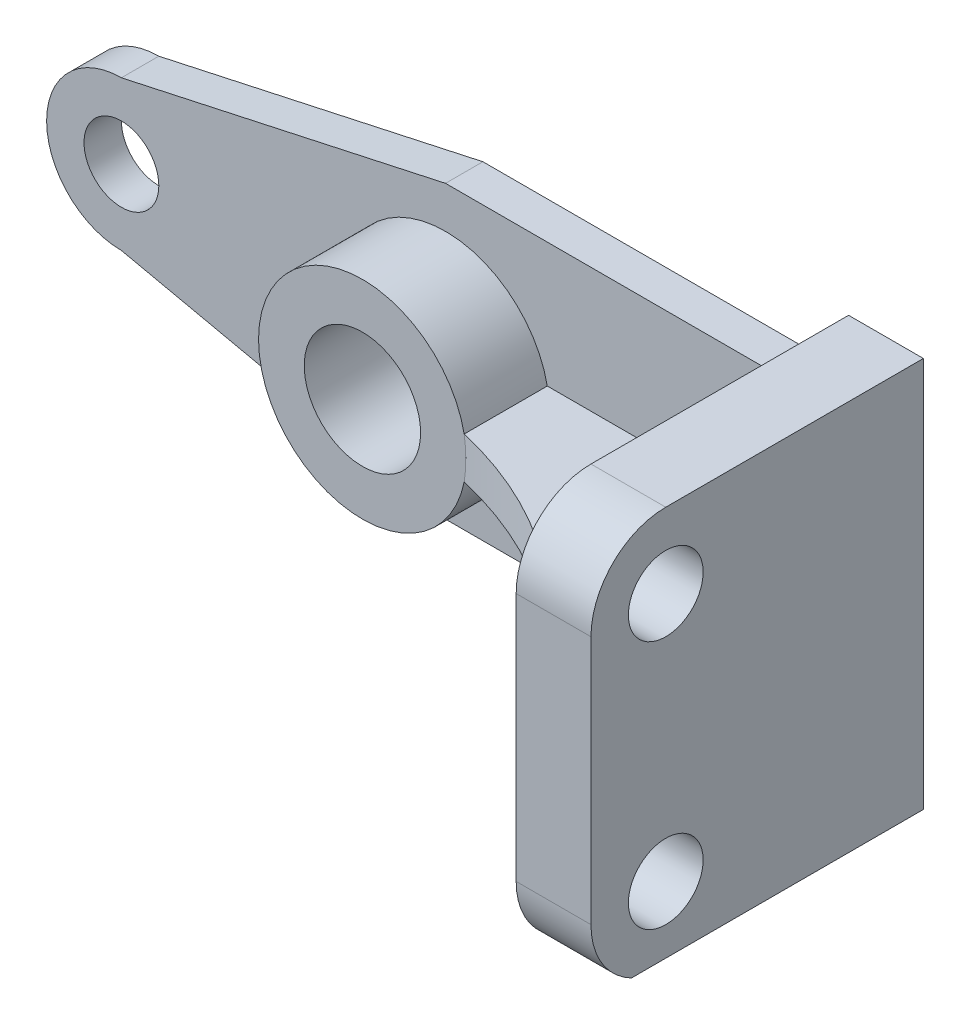
ISO-10303-21;
HEADER;
FILE_DESCRIPTION(('STEP AP214'),'2;1');
FILE_NAME('part.step','',(''),(''),'','','');
FILE_SCHEMA(('AUTOMOTIVE_DESIGN { 1 0 10303 214 1 1 1 1 }'));
ENDSEC;
DATA;
#1=APPLICATION_CONTEXT('core data for automotive mechanical design processes');
#2=APPLICATION_PROTOCOL_DEFINITION('international standard','automotive_design',2000,#1);
#3=PRODUCT_CONTEXT('',#1,'mechanical');
#4=PRODUCT('Part','Part','',(#3));
#5=PRODUCT_RELATED_PRODUCT_CATEGORY('part','',(#4));
#6=PRODUCT_DEFINITION_FORMATION('','',#4);
#7=PRODUCT_DEFINITION_CONTEXT('part definition',#1,'design');
#8=PRODUCT_DEFINITION('design','',#6,#7);
#9=PRODUCT_DEFINITION_SHAPE('','',#8);
#10=(LENGTH_UNIT() NAMED_UNIT(*) SI_UNIT(.MILLI.,.METRE.));
#11=(NAMED_UNIT(*) PLANE_ANGLE_UNIT() SI_UNIT($,.RADIAN.));
#12=(NAMED_UNIT(*) SI_UNIT($,.STERADIAN.) SOLID_ANGLE_UNIT());
#13=UNCERTAINTY_MEASURE_WITH_UNIT(LENGTH_MEASURE(1.E-05),#10,'distance_accuracy_value','');
#14=(GEOMETRIC_REPRESENTATION_CONTEXT(3) GLOBAL_UNCERTAINTY_ASSIGNED_CONTEXT((#13)) GLOBAL_UNIT_ASSIGNED_CONTEXT((#10,
#11,#12)) REPRESENTATION_CONTEXT('',''));
#15=CARTESIAN_POINT('',(0.,0.,0.));
#16=DIRECTION('',(0.,0.,1.));
#17=DIRECTION('',(1.,0.,0.));
#18=AXIS2_PLACEMENT_3D('',#15,#16,#17);
#19=CARTESIAN_POINT('',(88.,-30.9999999999999,62.));
#20=DIRECTION('',(-1.,0.,0.));
#21=DIRECTION('',(0.,0.,1.));
#22=AXIS2_PLACEMENT_3D('',#19,#20,#21);
#23=PLANE('',#22);
#24=CARTESIAN_POINT('',(88.,29.0000000000001,62.));
#25=DIRECTION('',(1.,0.,0.));
#26=DIRECTION('',(0.,0.,-1.));
#27=AXIS2_PLACEMENT_3D('',#24,#25,#26);
#28=CIRCLE('',#27,9.00000000000001);
#29=CARTESIAN_POINT('',(88.,29.0000000000001,53.));
#30=VERTEX_POINT('',#29);
#31=EDGE_CURVE('E407',#30,#30,#28,.T.);
#32=ORIENTED_EDGE('',*,*,#31,.T.);
#33=EDGE_LOOP('',(#32));
#34=FACE_BOUND('',#33,.T.);
#35=DIRECTION('',(0.,1.,0.));
#36=VECTOR('',#35,1.);
#37=CARTESIAN_POINT('',(88.,47.0000000000001,9.));
#38=LINE('',#37,#36);
#39=CARTESIAN_POINT('',(88.,5.,8.99999999999999));
#40=VERTEX_POINT('',#39);
#41=CARTESIAN_POINT('',(88.,47.0000000000001,9.));
#42=VERTEX_POINT('',#41);
#43=EDGE_CURVE('E185',#40,#42,#38,.T.);
#44=ORIENTED_EDGE('',*,*,#43,.F.);
#45=DIRECTION('',(0.,0.,-1.));
#46=VECTOR('',#45,1.);
#47=CARTESIAN_POINT('',(88.,5.,80.));
#48=LINE('',#47,#46);
#49=CARTESIAN_POINT('',(88.,5.,80.));
#50=VERTEX_POINT('',#49);
#51=EDGE_CURVE('E430',#50,#40,#48,.T.);
#52=ORIENTED_EDGE('',*,*,#51,.F.);
#53=DIRECTION('',(0.,-1.,0.));
#54=VECTOR('',#53,1.);
#55=CARTESIAN_POINT('',(88.,29.,80.));
#56=LINE('',#55,#54);
#57=CARTESIAN_POINT('',(88.,29.,80.));
#58=VERTEX_POINT('',#57);
#59=EDGE_CURVE('E392',#58,#50,#56,.T.);
#60=ORIENTED_EDGE('',*,*,#59,.F.);
#61=CARTESIAN_POINT('',(88.,29.0000000000001,62.));
#62=DIRECTION('',(1.,0.,0.));
#63=DIRECTION('',(0.,0.,-1.));
#64=AXIS2_PLACEMENT_3D('',#61,#62,#63);
#65=CIRCLE('',#64,18.);
#66=CARTESIAN_POINT('',(88.,47.0000000000001,61.9999999999999));
#67=VERTEX_POINT('',#66);
#68=EDGE_CURVE('E400',#67,#58,#65,.T.);
#69=ORIENTED_EDGE('',*,*,#68,.F.);
#70=DIRECTION('',(0.,0.,1.));
#71=VECTOR('',#70,1.);
#72=CARTESIAN_POINT('',(88.,47.0000000000001,9.));
#73=LINE('',#72,#71);
#74=EDGE_CURVE('E397',#42,#67,#73,.T.);
#75=ORIENTED_EDGE('',*,*,#74,.F.);
#76=EDGE_LOOP('',(#44,#52,#60,#69,#75));
#77=FACE_BOUND('',#76,.T.);
#78=ADVANCED_FACE('F43',(#34,#77),#23,.T.);
#79=CARTESIAN_POINT('',(0.,0.,9.));
#80=DIRECTION('',(0.,0.,1.));
#81=DIRECTION('',(1.,0.,0.));
#82=AXIS2_PLACEMENT_3D('',#79,#80,#81);
#83=PLANE('',#82);
#84=DIRECTION('',(-1.,0.,0.));
#85=VECTOR('',#84,1.);
#86=CARTESIAN_POINT('',(0.,-5.,9.));
#87=LINE('',#86,#85);
#88=CARTESIAN_POINT('',(88.,-5.,8.99999999999999));
#89=VERTEX_POINT('',#88);
#90=CARTESIAN_POINT('',(24.4948974278318,-5.,9.));
#91=VERTEX_POINT('',#90);
#92=EDGE_CURVE('E431',#89,#91,#87,.T.);
#93=ORIENTED_EDGE('',*,*,#92,.T.);
#94=CARTESIAN_POINT('',(0.,0.,9.));
#95=DIRECTION('',(0.,0.,1.));
#96=DIRECTION('',(1.,0.,0.));
#97=AXIS2_PLACEMENT_3D('',#94,#95,#96);
#98=CIRCLE('',#97,25.);
#99=CARTESIAN_POINT('',(24.4948974278318,5.,9.));
#100=VERTEX_POINT('',#99);
#101=EDGE_CURVE('E420',#100,#91,#98,.T.);
#102=ORIENTED_EDGE('',*,*,#101,.F.);
#103=DIRECTION('',(-1.,0.,0.));
#104=VECTOR('',#103,1.);
#105=CARTESIAN_POINT('',(0.,5.,9.));
#106=LINE('',#105,#104);
#107=EDGE_CURVE('E63',#40,#100,#106,.T.);
#108=ORIENTED_EDGE('',*,*,#107,.F.);
#109=ORIENTED_EDGE('',*,*,#43,.T.);
#110=CARTESIAN_POINT('',(76.,47.,9.));
#111=DIRECTION('',(0.,0.,1.));
#112=DIRECTION('',(1.,0.,0.));
#113=AXIS2_PLACEMENT_3D('',#110,#111,#112);
#114=CIRCLE('',#113,12.);
#115=CARTESIAN_POINT('',(75.9999999999999,35.,9.));
#116=VERTEX_POINT('',#115);
#117=EDGE_CURVE('E345',#116,#42,#114,.T.);
#118=ORIENTED_EDGE('',*,*,#117,.F.);
#119=DIRECTION('',(1.,0.,0.));
#120=VECTOR('',#119,1.);
#121=CARTESIAN_POINT('',(0.,35.,9.));
#122=LINE('',#121,#120);
#123=CARTESIAN_POINT('',(0.,35.,9.));
#124=VERTEX_POINT('',#123);
#125=EDGE_CURVE('E346',#124,#116,#122,.T.);
#126=ORIENTED_EDGE('',*,*,#125,.F.);
#127=DIRECTION('',(-0.977063170926614,-0.212949665458365,0.));
#128=VECTOR('',#127,1.);
#129=CARTESIAN_POINT('',(-7.2822846383179,33.412835399341,9.));
#130=LINE('',#129,#128);
#131=CARTESIAN_POINT('',(-78.,18.,9.));
#132=VERTEX_POINT('',#131);
#133=EDGE_CURVE('E348',#124,#132,#130,.T.);
#134=ORIENTED_EDGE('',*,*,#133,.T.);
#135=CARTESIAN_POINT('',(-78.,0.,9.));
#136=DIRECTION('',(0.,0.,1.));
#137=DIRECTION('',(1.,0.,0.));
#138=AXIS2_PLACEMENT_3D('',#135,#136,#137);
#139=CIRCLE('',#138,18.);
#140=CARTESIAN_POINT('',(-78.,-18.,9.));
#141=VERTEX_POINT('',#140);
#142=EDGE_CURVE('E354',#132,#141,#139,.T.);
#143=ORIENTED_EDGE('',*,*,#142,.T.);
#144=DIRECTION('',(0.977063170926614,-0.212949665458365,0.));
#145=VECTOR('',#144,1.);
#146=CARTESIAN_POINT('',(-7.2822846383179,-33.412835399341,9.));
#147=LINE('',#146,#145);
#148=CARTESIAN_POINT('',(0.,-35.,9.));
#149=VERTEX_POINT('',#148);
#150=EDGE_CURVE('E357',#141,#149,#147,.T.);
#151=ORIENTED_EDGE('',*,*,#150,.T.);
#152=DIRECTION('',(1.,0.,0.));
#153=VECTOR('',#152,1.);
#154=CARTESIAN_POINT('',(0.,-35.,9.));
#155=LINE('',#154,#153);
#156=CARTESIAN_POINT('',(75.9999999999999,-35.,9.));
#157=VERTEX_POINT('',#156);
#158=EDGE_CURVE('E186',#149,#157,#155,.T.);
#159=ORIENTED_EDGE('',*,*,#158,.T.);
#160=CARTESIAN_POINT('',(76.,-47.,9.));
#161=DIRECTION('',(0.,0.,1.));
#162=DIRECTION('',(1.,0.,0.));
#163=AXIS2_PLACEMENT_3D('',#160,#161,#162);
#164=CIRCLE('',#163,12.);
#165=CARTESIAN_POINT('',(88.,-47.0000000000001,8.99999999999999));
#166=VERTEX_POINT('',#165);
#167=EDGE_CURVE('E184',#157,#166,#164,.F.);
#168=ORIENTED_EDGE('',*,*,#167,.T.);
#169=EDGE_CURVE('E173',#166,#89,#38,.T.);
#170=ORIENTED_EDGE('',*,*,#169,.T.);
#171=EDGE_LOOP('',(#93,#102,#108,#109,#118,#126,#134,#143,#151,#159,#168,#170));
#172=FACE_BOUND('',#171,.T.);
#173=CARTESIAN_POINT('',(-78.,0.,9.));
#174=DIRECTION('',(0.,0.,1.));
#175=DIRECTION('',(1.,0.,0.));
#176=AXIS2_PLACEMENT_3D('',#173,#174,#175);
#177=CIRCLE('',#176,9.);
#178=CARTESIAN_POINT('',(-69.,0.,9.));
#179=VERTEX_POINT('',#178);
#180=EDGE_CURVE('E194',#179,#179,#177,.T.);
#181=ORIENTED_EDGE('',*,*,#180,.F.);
#182=EDGE_LOOP('',(#181));
#183=FACE_BOUND('',#182,.T.);
#184=ADVANCED_FACE('F187',(#172,#183),#83,.T.);
#185=CARTESIAN_POINT('',(76.,47.,9.));
#186=DIRECTION('',(0.,0.,-1.));
#187=DIRECTION('',(-1.,0.,0.));
#188=AXIS2_PLACEMENT_3D('',#185,#186,#187);
#189=CYLINDRICAL_SURFACE('',#188,12.);
#190=CARTESIAN_POINT('',(76.,47.,0.));
#191=DIRECTION('',(0.,0.,1.));
#192=DIRECTION('',(1.,0.,0.));
#193=AXIS2_PLACEMENT_3D('',#190,#191,#192);
#194=CIRCLE('',#193,12.);
#195=CARTESIAN_POINT('',(75.9999999999999,35.,0.));
#196=VERTEX_POINT('',#195);
#197=CARTESIAN_POINT('',(88.,47.0000000000001,0.));
#198=VERTEX_POINT('',#197);
#199=EDGE_CURVE('E321',#196,#198,#194,.T.);
#200=ORIENTED_EDGE('',*,*,#199,.F.);
#201=DIRECTION('',(0.,0.,-1.));
#202=VECTOR('',#201,1.);
#203=CARTESIAN_POINT('',(75.9999999999999,35.,9.));
#204=LINE('',#203,#202);
#205=EDGE_CURVE('E220',#116,#196,#204,.T.);
#206=ORIENTED_EDGE('',*,*,#205,.F.);
#207=ORIENTED_EDGE('',*,*,#117,.T.);
#208=DIRECTION('',(0.,0.,-1.));
#209=VECTOR('',#208,1.);
#210=CARTESIAN_POINT('',(88.,47.0000000000001,9.));
#211=LINE('',#210,#209);
#212=EDGE_CURVE('E198',#42,#198,#211,.T.);
#213=ORIENTED_EDGE('',*,*,#212,.T.);
#214=EDGE_LOOP('',(#200,#206,#207,#213));
#215=FACE_BOUND('',#214,.T.);
#216=ADVANCED_FACE('F44',(#215),#189,.F.);
#217=CARTESIAN_POINT('',(0.,35.,9.));
#218=DIRECTION('',(0.,1.,0.));
#219=DIRECTION('',(-1.,0.,0.));
#220=AXIS2_PLACEMENT_3D('',#217,#218,#219);
#221=PLANE('',#220);
#222=DIRECTION('',(1.,0.,0.));
#223=VECTOR('',#222,1.);
#224=CARTESIAN_POINT('',(0.,35.,0.));
#225=LINE('',#224,#223);
#226=CARTESIAN_POINT('',(0.,35.,0.));
#227=VERTEX_POINT('',#226);
#228=EDGE_CURVE('E320',#227,#196,#225,.T.);
#229=ORIENTED_EDGE('',*,*,#228,.F.);
#230=DIRECTION('',(0.,0.,-1.));
#231=VECTOR('',#230,1.);
#232=CARTESIAN_POINT('',(0.,35.,9.));
#233=LINE('',#232,#231);
#234=EDGE_CURVE('E213',#124,#227,#233,.T.);
#235=ORIENTED_EDGE('',*,*,#234,.F.);
#236=ORIENTED_EDGE('',*,*,#125,.T.);
#237=ORIENTED_EDGE('',*,*,#205,.T.);
#238=EDGE_LOOP('',(#229,#235,#236,#237));
#239=FACE_BOUND('',#238,.T.);
#240=ADVANCED_FACE('F310',(#239),#221,.T.);
#241=CARTESIAN_POINT('',(-7.2822846383179,33.412835399341,9.));
#242=DIRECTION('',(0.212949665458365,-0.977063170926614,0.));
#243=DIRECTION('',(0.977063170926615,0.212949665458365,0.));
#244=AXIS2_PLACEMENT_3D('',#241,#242,#243);
#245=PLANE('',#244);
#246=DIRECTION('',(-0.977063170926614,-0.212949665458365,0.));
#247=VECTOR('',#246,1.);
#248=CARTESIAN_POINT('',(-7.2822846383179,33.412835399341,0.));
#249=LINE('',#248,#247);
#250=CARTESIAN_POINT('',(-78.,18.,0.));
#251=VERTEX_POINT('',#250);
#252=EDGE_CURVE('E324',#227,#251,#249,.T.);
#253=ORIENTED_EDGE('',*,*,#252,.T.);
#254=DIRECTION('',(0.,0.,-1.));
#255=VECTOR('',#254,1.);
#256=CARTESIAN_POINT('',(-78.,18.,9.));
#257=LINE('',#256,#255);
#258=EDGE_CURVE('E215',#132,#251,#257,.T.);
#259=ORIENTED_EDGE('',*,*,#258,.F.);
#260=ORIENTED_EDGE('',*,*,#133,.F.);
#261=ORIENTED_EDGE('',*,*,#234,.T.);
#262=EDGE_LOOP('',(#253,#259,#260,#261));
#263=FACE_BOUND('',#262,.T.);
#264=ADVANCED_FACE('F302',(#263),#245,.F.);
#265=CARTESIAN_POINT('',(-78.,0.,9.));
#266=DIRECTION('',(0.,0.,-1.));
#267=DIRECTION('',(-1.,0.,0.));
#268=AXIS2_PLACEMENT_3D('',#265,#266,#267);
#269=CYLINDRICAL_SURFACE('',#268,18.);
#270=CARTESIAN_POINT('',(-78.,0.,0.));
#271=DIRECTION('',(0.,0.,1.));
#272=DIRECTION('',(1.,0.,0.));
#273=AXIS2_PLACEMENT_3D('',#270,#271,#272);
#274=CIRCLE('',#273,18.);
#275=CARTESIAN_POINT('',(-78.,-18.,0.));
#276=VERTEX_POINT('',#275);
#277=EDGE_CURVE('E326',#251,#276,#274,.T.);
#278=ORIENTED_EDGE('',*,*,#277,.T.);
#279=DIRECTION('',(0.,0.,-1.));
#280=VECTOR('',#279,1.);
#281=CARTESIAN_POINT('',(-78.,-18.,9.));
#282=LINE('',#281,#280);
#283=EDGE_CURVE('E209',#141,#276,#282,.T.);
#284=ORIENTED_EDGE('',*,*,#283,.F.);
#285=ORIENTED_EDGE('',*,*,#142,.F.);
#286=ORIENTED_EDGE('',*,*,#258,.T.);
#287=EDGE_LOOP('',(#278,#284,#285,#286));
#288=FACE_BOUND('',#287,.T.);
#289=ADVANCED_FACE('F297',(#288),#269,.T.);
#290=CARTESIAN_POINT('',(-7.2822846383179,-33.412835399341,9.));
#291=DIRECTION('',(0.212949665458365,0.977063170926614,0.));
#292=DIRECTION('',(-0.977063170926615,0.212949665458365,0.));
#293=AXIS2_PLACEMENT_3D('',#290,#291,#292);
#294=PLANE('',#293);
#295=DIRECTION('',(0.977063170926614,-0.212949665458365,0.));
#296=VECTOR('',#295,1.);
#297=CARTESIAN_POINT('',(-7.2822846383179,-33.412835399341,0.));
#298=LINE('',#297,#296);
#299=CARTESIAN_POINT('',(0.,-35.,0.));
#300=VERTEX_POINT('',#299);
#301=EDGE_CURVE('E331',#276,#300,#298,.T.);
#302=ORIENTED_EDGE('',*,*,#301,.T.);
#303=DIRECTION('',(0.,0.,-1.));
#304=VECTOR('',#303,1.);
#305=CARTESIAN_POINT('',(0.,-35.,9.));
#306=LINE('',#305,#304);
#307=EDGE_CURVE('E203',#149,#300,#306,.T.);
#308=ORIENTED_EDGE('',*,*,#307,.F.);
#309=ORIENTED_EDGE('',*,*,#150,.F.);
#310=ORIENTED_EDGE('',*,*,#283,.T.);
#311=EDGE_LOOP('',(#302,#308,#309,#310));
#312=FACE_BOUND('',#311,.T.);
#313=ADVANCED_FACE('F298',(#312),#294,.F.);
#314=CARTESIAN_POINT('',(0.,-35.,9.));
#315=DIRECTION('',(0.,1.,0.));
#316=DIRECTION('',(0.,0.,1.));
#317=AXIS2_PLACEMENT_3D('',#314,#315,#316);
#318=PLANE('',#317);
#319=DIRECTION('',(1.,0.,0.));
#320=VECTOR('',#319,1.);
#321=CARTESIAN_POINT('',(0.,-35.,0.));
#322=LINE('',#321,#320);
#323=CARTESIAN_POINT('',(75.9999999999999,-35.,0.));
#324=VERTEX_POINT('',#323);
#325=EDGE_CURVE('E334',#300,#324,#322,.T.);
#326=ORIENTED_EDGE('',*,*,#325,.T.);
#327=DIRECTION('',(0.,0.,-1.));
#328=VECTOR('',#327,1.);
#329=CARTESIAN_POINT('',(75.9999999999999,-35.,9.));
#330=LINE('',#329,#328);
#331=EDGE_CURVE('E197',#157,#324,#330,.T.);
#332=ORIENTED_EDGE('',*,*,#331,.F.);
#333=ORIENTED_EDGE('',*,*,#158,.F.);
#334=ORIENTED_EDGE('',*,*,#307,.T.);
#335=EDGE_LOOP('',(#326,#332,#333,#334));
#336=FACE_BOUND('',#335,.T.);
#337=ADVANCED_FACE('F291',(#336),#318,.F.);
#338=CARTESIAN_POINT('',(76.,-47.,9.));
#339=DIRECTION('',(0.,0.,-1.));
#340=DIRECTION('',(-1.,0.,0.));
#341=AXIS2_PLACEMENT_3D('',#338,#339,#340);
#342=CYLINDRICAL_SURFACE('',#341,12.);
#343=CARTESIAN_POINT('',(76.,-47.,0.));
#344=DIRECTION('',(0.,0.,1.));
#345=DIRECTION('',(1.,0.,0.));
#346=AXIS2_PLACEMENT_3D('',#343,#344,#345);
#347=CIRCLE('',#346,12.);
#348=CARTESIAN_POINT('',(88.,-47.0000000000001,0.));
#349=VERTEX_POINT('',#348);
#350=EDGE_CURVE('E200',#324,#349,#347,.F.);
#351=ORIENTED_EDGE('',*,*,#350,.T.);
#352=DIRECTION('',(0.,0.,-1.));
#353=VECTOR('',#352,1.);
#354=CARTESIAN_POINT('',(88.,-47.0000000000001,9.));
#355=LINE('',#354,#353);
#356=EDGE_CURVE('E164',#166,#349,#355,.T.);
#357=ORIENTED_EDGE('',*,*,#356,.F.);
#358=ORIENTED_EDGE('',*,*,#167,.F.);
#359=ORIENTED_EDGE('',*,*,#331,.T.);
#360=EDGE_LOOP('',(#351,#357,#358,#359));
#361=FACE_BOUND('',#360,.T.);
#362=ADVANCED_FACE('F193',(#361),#342,.F.);
#363=CARTESIAN_POINT('',(0.,0.,9.));
#364=DIRECTION('',(0.,0.,-1.));
#365=DIRECTION('',(-1.,0.,0.));
#366=AXIS2_PLACEMENT_3D('',#363,#364,#365);
#367=CYLINDRICAL_SURFACE('',#366,14.);
#368=CARTESIAN_POINT('',(0.,0.,0.));
#369=DIRECTION('',(0.,0.,1.));
#370=DIRECTION('',(1.,0.,0.));
#371=AXIS2_PLACEMENT_3D('',#368,#369,#370);
#372=CIRCLE('',#371,14.);
#373=CARTESIAN_POINT('',(14.,0.,0.));
#374=VERTEX_POINT('',#373);
#375=EDGE_CURVE('E336',#374,#374,#372,.T.);
#376=ORIENTED_EDGE('',*,*,#375,.F.);
#377=EDGE_LOOP('',(#376));
#378=FACE_BOUND('',#377,.T.);
#379=CARTESIAN_POINT('',(0.,0.,29.));
#380=DIRECTION('',(0.,0.,1.));
#381=DIRECTION('',(1.,0.,0.));
#382=AXIS2_PLACEMENT_3D('',#379,#380,#381);
#383=CIRCLE('',#382,14.);
#384=CARTESIAN_POINT('',(14.,0.,29.));
#385=VERTEX_POINT('',#384);
#386=EDGE_CURVE('E423',#385,#385,#383,.T.);
#387=ORIENTED_EDGE('',*,*,#386,.T.);
#388=EDGE_LOOP('',(#387));
#389=FACE_BOUND('',#388,.T.);
#390=ADVANCED_FACE('F290',(#378,#389),#367,.F.);
#391=CARTESIAN_POINT('',(-78.,0.,9.));
#392=DIRECTION('',(0.,0.,-1.));
#393=DIRECTION('',(-1.,0.,0.));
#394=AXIS2_PLACEMENT_3D('',#391,#392,#393);
#395=CYLINDRICAL_SURFACE('',#394,9.);
#396=ORIENTED_EDGE('',*,*,#180,.T.);
#397=EDGE_LOOP('',(#396));
#398=FACE_BOUND('',#397,.T.);
#399=CARTESIAN_POINT('',(-78.,0.,0.));
#400=DIRECTION('',(0.,0.,1.));
#401=DIRECTION('',(1.,0.,0.));
#402=AXIS2_PLACEMENT_3D('',#399,#400,#401);
#403=CIRCLE('',#402,9.);
#404=CARTESIAN_POINT('',(-69.,0.,0.));
#405=VERTEX_POINT('',#404);
#406=EDGE_CURVE('E338',#405,#405,#403,.T.);
#407=ORIENTED_EDGE('',*,*,#406,.F.);
#408=EDGE_LOOP('',(#407));
#409=FACE_BOUND('',#408,.T.);
#410=ADVANCED_FACE('F282',(#398,#409),#395,.F.);
#411=CARTESIAN_POINT('',(0.,0.,0.));
#412=DIRECTION('',(0.,0.,1.));
#413=DIRECTION('',(1.,0.,0.));
#414=AXIS2_PLACEMENT_3D('',#411,#412,#413);
#415=PLANE('',#414);
#416=ORIENTED_EDGE('',*,*,#199,.T.);
#417=DIRECTION('',(-1.,0.,0.));
#418=VECTOR('',#417,1.);
#419=CARTESIAN_POINT('',(106.,47.0000000000001,0.));
#420=LINE('',#419,#418);
#421=CARTESIAN_POINT('',(106.,47.0000000000001,0.));
#422=VERTEX_POINT('',#421);
#423=EDGE_CURVE('E375',#422,#198,#420,.T.);
#424=ORIENTED_EDGE('',*,*,#423,.F.);
#425=DIRECTION('',(0.,1.,0.));
#426=VECTOR('',#425,1.);
#427=CARTESIAN_POINT('',(106.,47.0000000000001,0.));
#428=LINE('',#427,#426);
#429=CARTESIAN_POINT('',(106.,-47.0000000000001,0.));
#430=VERTEX_POINT('',#429);
#431=EDGE_CURVE('E371',#430,#422,#428,.T.);
#432=ORIENTED_EDGE('',*,*,#431,.F.);
#433=DIRECTION('',(-1.,0.,0.));
#434=VECTOR('',#433,1.);
#435=CARTESIAN_POINT('',(106.,-47.0000000000001,0.));
#436=LINE('',#435,#434);
#437=EDGE_CURVE('E327',#430,#349,#436,.T.);
#438=ORIENTED_EDGE('',*,*,#437,.T.);
#439=ORIENTED_EDGE('',*,*,#350,.F.);
#440=ORIENTED_EDGE('',*,*,#325,.F.);
#441=ORIENTED_EDGE('',*,*,#301,.F.);
#442=ORIENTED_EDGE('',*,*,#277,.F.);
#443=ORIENTED_EDGE('',*,*,#252,.F.);
#444=ORIENTED_EDGE('',*,*,#228,.T.);
#445=EDGE_LOOP('',(#416,#424,#432,#438,#439,#440,#441,#442,#443,#444));
#446=FACE_BOUND('',#445,.T.);
#447=ORIENTED_EDGE('',*,*,#375,.T.);
#448=EDGE_LOOP('',(#447));
#449=FACE_BOUND('',#448,.T.);
#450=ORIENTED_EDGE('',*,*,#406,.T.);
#451=EDGE_LOOP('',(#450));
#452=FACE_BOUND('',#451,.T.);
#453=ADVANCED_FACE('F276',(#446,#449,#452),#415,.F.);
#454=CARTESIAN_POINT('',(106.,-47.0000000000001,9.));
#455=DIRECTION('',(0.,1.,0.));
#456=DIRECTION('',(0.,0.,1.));
#457=AXIS2_PLACEMENT_3D('',#454,#455,#456);
#458=PLANE('',#457);
#459=ORIENTED_EDGE('',*,*,#356,.T.);
#460=ORIENTED_EDGE('',*,*,#437,.F.);
#461=DIRECTION('',(0.,0.,-1.));
#462=VECTOR('',#461,1.);
#463=CARTESIAN_POINT('',(106.,-47.0000000000001,9.));
#464=LINE('',#463,#462);
#465=CARTESIAN_POINT('',(106.,-47.0000000000001,70.2462112512349));
#466=VERTEX_POINT('',#465);
#467=EDGE_CURVE('E59',#466,#430,#464,.T.);
#468=ORIENTED_EDGE('',*,*,#467,.F.);
#469=DIRECTION('',(-1.,0.,0.));
#470=VECTOR('',#469,1.);
#471=CARTESIAN_POINT('',(106.,-47.0000000000001,70.2462112512349));
#472=LINE('',#471,#470);
#473=CARTESIAN_POINT('',(88.,-47.0000000000001,70.2462112512349));
#474=VERTEX_POINT('',#473);
#475=EDGE_CURVE('E11',#474,#466,#472,.F.);
#476=ORIENTED_EDGE('',*,*,#475,.F.);
#477=DIRECTION('',(0.,0.,-1.));
#478=VECTOR('',#477,1.);
#479=CARTESIAN_POINT('',(88.,-47.0000000000001,80.));
#480=LINE('',#479,#478);
#481=EDGE_CURVE('E163',#474,#166,#480,.T.);
#482=ORIENTED_EDGE('',*,*,#481,.T.);
#483=EDGE_LOOP('',(#459,#460,#468,#476,#482));
#484=FACE_BOUND('',#483,.T.);
#485=ADVANCED_FACE('F161',(#484),#458,.F.);
#486=CARTESIAN_POINT('',(106.,47.0000000000001,9.));
#487=DIRECTION('',(0.,-1.,0.));
#488=DIRECTION('',(0.,0.,-1.));
#489=AXIS2_PLACEMENT_3D('',#486,#487,#488);
#490=PLANE('',#489);
#491=ORIENTED_EDGE('',*,*,#212,.F.);
#492=ORIENTED_EDGE('',*,*,#74,.T.);
#493=DIRECTION('',(-1.,0.,0.));
#494=VECTOR('',#493,1.);
#495=CARTESIAN_POINT('',(106.,47.0000000000001,61.9999999999999));
#496=LINE('',#495,#494);
#497=CARTESIAN_POINT('',(106.,47.0000000000001,61.9999999999999));
#498=VERTEX_POINT('',#497);
#499=EDGE_CURVE('E379',#498,#67,#496,.T.);
#500=ORIENTED_EDGE('',*,*,#499,.F.);
#501=DIRECTION('',(0.,0.,1.));
#502=VECTOR('',#501,1.);
#503=CARTESIAN_POINT('',(106.,47.0000000000001,9.));
#504=LINE('',#503,#502);
#505=EDGE_CURVE('E373',#422,#498,#504,.T.);
#506=ORIENTED_EDGE('',*,*,#505,.F.);
#507=ORIENTED_EDGE('',*,*,#423,.T.);
#508=EDGE_LOOP('',(#491,#492,#500,#506,#507));
#509=FACE_BOUND('',#508,.T.);
#510=ADVANCED_FACE('F268',(#509),#490,.F.);
#511=CARTESIAN_POINT('',(106.,0.,0.));
#512=DIRECTION('',(1.,0.,0.));
#513=DIRECTION('',(0.,0.,-1.));
#514=AXIS2_PLACEMENT_3D('',#511,#512,#513);
#515=PLANE('',#514);
#516=CARTESIAN_POINT('',(106.,-30.9999999999999,62.));
#517=DIRECTION('',(1.,0.,0.));
#518=DIRECTION('',(0.,0.,1.));
#519=AXIS2_PLACEMENT_3D('',#516,#517,#518);
#520=CIRCLE('',#519,18.);
#521=CARTESIAN_POINT('',(106.,-30.9999999999998,80.));
#522=VERTEX_POINT('',#521);
#523=EDGE_CURVE('E386',#522,#466,#520,.T.);
#524=ORIENTED_EDGE('',*,*,#523,.T.);
#525=ORIENTED_EDGE('',*,*,#467,.T.);
#526=ORIENTED_EDGE('',*,*,#431,.T.);
#527=ORIENTED_EDGE('',*,*,#505,.T.);
#528=CARTESIAN_POINT('',(106.,29.0000000000001,62.));
#529=DIRECTION('',(1.,0.,0.));
#530=DIRECTION('',(0.,0.,-1.));
#531=AXIS2_PLACEMENT_3D('',#528,#529,#530);
#532=CIRCLE('',#531,18.);
#533=CARTESIAN_POINT('',(106.,29.,80.));
#534=VERTEX_POINT('',#533);
#535=EDGE_CURVE('E395',#498,#534,#532,.T.);
#536=ORIENTED_EDGE('',*,*,#535,.T.);
#537=DIRECTION('',(0.,-1.,0.));
#538=VECTOR('',#537,1.);
#539=CARTESIAN_POINT('',(106.,29.,80.));
#540=LINE('',#539,#538);
#541=EDGE_CURVE('E401',#534,#522,#540,.T.);
#542=ORIENTED_EDGE('',*,*,#541,.T.);
#543=EDGE_LOOP('',(#524,#525,#526,#527,#536,#542));
#544=FACE_BOUND('',#543,.T.);
#545=CARTESIAN_POINT('',(106.,29.0000000000001,62.));
#546=DIRECTION('',(1.,0.,0.));
#547=DIRECTION('',(0.,0.,-1.));
#548=AXIS2_PLACEMENT_3D('',#545,#546,#547);
#549=CIRCLE('',#548,9.00000000000001);
#550=CARTESIAN_POINT('',(106.,29.0000000000001,53.));
#551=VERTEX_POINT('',#550);
#552=EDGE_CURVE('E399',#551,#551,#549,.T.);
#553=ORIENTED_EDGE('',*,*,#552,.F.);
#554=EDGE_LOOP('',(#553));
#555=FACE_BOUND('',#554,.T.);
#556=CARTESIAN_POINT('',(106.,-30.9999999999999,62.));
#557=DIRECTION('',(1.,0.,0.));
#558=DIRECTION('',(0.,0.,-1.));
#559=AXIS2_PLACEMENT_3D('',#556,#557,#558);
#560=CIRCLE('',#559,9.);
#561=CARTESIAN_POINT('',(106.,-30.9999999999999,53.));
#562=VERTEX_POINT('',#561);
#563=EDGE_CURVE('E409',#562,#562,#560,.T.);
#564=ORIENTED_EDGE('',*,*,#563,.F.);
#565=EDGE_LOOP('',(#564));
#566=FACE_BOUND('',#565,.T.);
#567=ADVANCED_FACE('F260',(#544,#555,#566),#515,.T.);
#568=ORIENTED_EDGE('',*,*,#481,.F.);
#569=CARTESIAN_POINT('',(88.,-30.9999999999999,62.));
#570=DIRECTION('',(1.,0.,0.));
#571=DIRECTION('',(0.,0.,1.));
#572=AXIS2_PLACEMENT_3D('',#569,#570,#571);
#573=CIRCLE('',#572,18.);
#574=CARTESIAN_POINT('',(88.,-30.9999999999998,80.));
#575=VERTEX_POINT('',#574);
#576=EDGE_CURVE('E388',#575,#474,#573,.T.);
#577=ORIENTED_EDGE('',*,*,#576,.F.);
#578=CARTESIAN_POINT('',(88.,-5.,80.));
#579=VERTEX_POINT('',#578);
#580=EDGE_CURVE('E398',#579,#575,#56,.T.);
#581=ORIENTED_EDGE('',*,*,#580,.F.);
#582=DIRECTION('',(0.,0.,-1.));
#583=VECTOR('',#582,1.);
#584=CARTESIAN_POINT('',(88.,-5.,80.));
#585=LINE('',#584,#583);
#586=EDGE_CURVE('E177',#579,#89,#585,.T.);
#587=ORIENTED_EDGE('',*,*,#586,.T.);
#588=ORIENTED_EDGE('',*,*,#169,.F.);
#589=EDGE_LOOP('',(#568,#577,#581,#587,#588));
#590=FACE_BOUND('',#589,.T.);
#591=CARTESIAN_POINT('',(88.,-30.9999999999999,62.));
#592=DIRECTION('',(1.,0.,0.));
#593=DIRECTION('',(0.,0.,-1.));
#594=AXIS2_PLACEMENT_3D('',#591,#592,#593);
#595=CIRCLE('',#594,9.);
#596=CARTESIAN_POINT('',(88.,-30.9999999999999,53.));
#597=VERTEX_POINT('',#596);
#598=EDGE_CURVE('E411',#597,#597,#595,.T.);
#599=ORIENTED_EDGE('',*,*,#598,.T.);
#600=EDGE_LOOP('',(#599));
#601=FACE_BOUND('',#600,.T.);
#602=ADVANCED_FACE('F174',(#590,#601),#23,.T.);
#603=CARTESIAN_POINT('',(106.,29.0000000000001,62.));
#604=DIRECTION('',(-1.,0.,0.));
#605=DIRECTION('',(0.,0.,1.));
#606=AXIS2_PLACEMENT_3D('',#603,#604,#605);
#607=CYLINDRICAL_SURFACE('',#606,18.);
#608=ORIENTED_EDGE('',*,*,#68,.T.);
#609=DIRECTION('',(-1.,0.,0.));
#610=VECTOR('',#609,1.);
#611=CARTESIAN_POINT('',(106.,29.,80.));
#612=LINE('',#611,#610);
#613=EDGE_CURVE('E384',#534,#58,#612,.T.);
#614=ORIENTED_EDGE('',*,*,#613,.F.);
#615=ORIENTED_EDGE('',*,*,#535,.F.);
#616=ORIENTED_EDGE('',*,*,#499,.T.);
#617=EDGE_LOOP('',(#608,#614,#615,#616));
#618=FACE_BOUND('',#617,.T.);
#619=ADVANCED_FACE('F257',(#618),#607,.T.);
#620=CARTESIAN_POINT('',(106.,29.,80.));
#621=DIRECTION('',(0.,0.,-1.));
#622=DIRECTION('',(0.,1.,0.));
#623=AXIS2_PLACEMENT_3D('',#620,#621,#622);
#624=PLANE('',#623);
#625=ORIENTED_EDGE('',*,*,#59,.T.);
#626=DIRECTION('',(0.,-1.,0.));
#627=VECTOR('',#626,1.);
#628=CARTESIAN_POINT('',(88.,47.0000000000001,80.));
#629=LINE('',#628,#627);
#630=EDGE_CURVE('E436',#50,#579,#629,.T.);
#631=ORIENTED_EDGE('',*,*,#630,.T.);
#632=ORIENTED_EDGE('',*,*,#580,.T.);
#633=DIRECTION('',(-1.,0.,0.));
#634=VECTOR('',#633,1.);
#635=CARTESIAN_POINT('',(106.,-30.9999999999998,80.));
#636=LINE('',#635,#634);
#637=EDGE_CURVE('E387',#522,#575,#636,.T.);
#638=ORIENTED_EDGE('',*,*,#637,.F.);
#639=ORIENTED_EDGE('',*,*,#541,.F.);
#640=ORIENTED_EDGE('',*,*,#613,.T.);
#641=EDGE_LOOP('',(#625,#631,#632,#638,#639,#640));
#642=FACE_BOUND('',#641,.T.);
#643=ADVANCED_FACE('F262',(#642),#624,.F.);
#644=CARTESIAN_POINT('',(106.,-30.9999999999999,62.));
#645=DIRECTION('',(-1.,0.,0.));
#646=DIRECTION('',(0.,0.,1.));
#647=AXIS2_PLACEMENT_3D('',#644,#645,#646);
#648=CYLINDRICAL_SURFACE('',#647,18.);
#649=ORIENTED_EDGE('',*,*,#576,.T.);
#650=ORIENTED_EDGE('',*,*,#475,.T.);
#651=ORIENTED_EDGE('',*,*,#523,.F.);
#652=ORIENTED_EDGE('',*,*,#637,.T.);
#653=EDGE_LOOP('',(#649,#650,#651,#652));
#654=FACE_BOUND('',#653,.T.);
#655=ADVANCED_FACE('F461',(#654),#648,.T.);
#656=CARTESIAN_POINT('',(106.,29.0000000000001,62.));
#657=DIRECTION('',(-1.,0.,0.));
#658=DIRECTION('',(0.,0.,1.));
#659=AXIS2_PLACEMENT_3D('',#656,#657,#658);
#660=CYLINDRICAL_SURFACE('',#659,9.00000000000001);
#661=ORIENTED_EDGE('',*,*,#552,.T.);
#662=EDGE_LOOP('',(#661));
#663=FACE_BOUND('',#662,.T.);
#664=ORIENTED_EDGE('',*,*,#31,.F.);
#665=EDGE_LOOP('',(#664));
#666=FACE_BOUND('',#665,.T.);
#667=ADVANCED_FACE('F462',(#663,#666),#660,.F.);
#668=CARTESIAN_POINT('',(106.,-30.9999999999999,62.));
#669=DIRECTION('',(-1.,0.,0.));
#670=DIRECTION('',(0.,0.,1.));
#671=AXIS2_PLACEMENT_3D('',#668,#669,#670);
#672=CYLINDRICAL_SURFACE('',#671,9.);
#673=ORIENTED_EDGE('',*,*,#563,.T.);
#674=EDGE_LOOP('',(#673));
#675=FACE_BOUND('',#674,.T.);
#676=ORIENTED_EDGE('',*,*,#598,.F.);
#677=EDGE_LOOP('',(#676));
#678=FACE_BOUND('',#677,.T.);
#679=ADVANCED_FACE('F466',(#675,#678),#672,.F.);
#680=CARTESIAN_POINT('',(0.,0.,29.));
#681=DIRECTION('',(0.,0.,1.));
#682=DIRECTION('',(1.,0.,0.));
#683=AXIS2_PLACEMENT_3D('',#680,#681,#682);
#684=PLANE('',#683);
#685=CARTESIAN_POINT('',(0.,0.,29.));
#686=DIRECTION('',(0.,0.,1.));
#687=DIRECTION('',(1.,0.,0.));
#688=AXIS2_PLACEMENT_3D('',#685,#686,#687);
#689=CIRCLE('',#688,25.);
#690=CARTESIAN_POINT('',(24.4948974278318,5.,29.));
#691=VERTEX_POINT('',#690);
#692=CARTESIAN_POINT('',(24.4948974278318,-5.,29.));
#693=VERTEX_POINT('',#692);
#694=EDGE_CURVE('E413',#691,#693,#689,.T.);
#695=ORIENTED_EDGE('',*,*,#694,.T.);
#696=EDGE_CURVE('E419',#693,#691,#689,.T.);
#697=ORIENTED_EDGE('',*,*,#696,.T.);
#698=EDGE_LOOP('',(#695,#697));
#699=FACE_BOUND('',#698,.T.);
#700=ORIENTED_EDGE('',*,*,#386,.F.);
#701=EDGE_LOOP('',(#700));
#702=FACE_BOUND('',#701,.T.);
#703=ADVANCED_FACE('F480',(#699,#702),#684,.T.);
#704=CARTESIAN_POINT('',(0.,0.,29.));
#705=DIRECTION('',(0.,0.,-1.));
#706=DIRECTION('',(-1.,0.,0.));
#707=AXIS2_PLACEMENT_3D('',#704,#705,#706);
#708=CYLINDRICAL_SURFACE('',#707,25.);
#709=ORIENTED_EDGE('',*,*,#101,.T.);
#710=DIRECTION('',(0.,0.,-1.));
#711=VECTOR('',#710,1.);
#712=CARTESIAN_POINT('',(24.4948974278318,-5.,29.));
#713=LINE('',#712,#711);
#714=EDGE_CURVE('E223',#91,#693,#713,.F.);
#715=ORIENTED_EDGE('',*,*,#714,.T.);
#716=ORIENTED_EDGE('',*,*,#694,.F.);
#717=DIRECTION('',(0.,0.,-1.));
#718=VECTOR('',#717,1.);
#719=CARTESIAN_POINT('',(24.4948974278318,5.,29.));
#720=LINE('',#719,#718);
#721=EDGE_CURVE('E181',#100,#691,#720,.F.);
#722=ORIENTED_EDGE('',*,*,#721,.F.);
#723=EDGE_LOOP('',(#709,#715,#716,#722));
#724=FACE_BOUND('',#723,.T.);
#725=ADVANCED_FACE('F450',(#724),#708,.T.);
#726=CARTESIAN_POINT('',(0.,-5.,80.));
#727=DIRECTION('',(0.,-1.,0.));
#728=DIRECTION('',(1.,0.,0.));
#729=AXIS2_PLACEMENT_3D('',#726,#727,#728);
#730=PLANE('',#729);
#731=CARTESIAN_POINT('',(3.19894347588805,-5.,120.555897381199));
#732=DIRECTION('',(0.,-1.,0.));
#733=DIRECTION('',(1.,0.,0.));
#734=AXIS2_PLACEMENT_3D('',#731,#732,#733);
#735=CIRCLE('',#734,94.);
#736=EDGE_CURVE('E167',#693,#579,#735,.T.);
#737=ORIENTED_EDGE('',*,*,#736,.F.);
#738=ORIENTED_EDGE('',*,*,#714,.F.);
#739=ORIENTED_EDGE('',*,*,#92,.F.);
#740=ORIENTED_EDGE('',*,*,#586,.F.);
#741=EDGE_LOOP('',(#737,#738,#739,#740));
#742=FACE_BOUND('',#741,.T.);
#743=ADVANCED_FACE('F444',(#742),#730,.T.);
#744=CARTESIAN_POINT('',(0.,5.,80.));
#745=DIRECTION('',(0.,-1.,0.));
#746=DIRECTION('',(1.,0.,0.));
#747=AXIS2_PLACEMENT_3D('',#744,#745,#746);
#748=PLANE('',#747);
#749=ORIENTED_EDGE('',*,*,#721,.T.);
#750=CARTESIAN_POINT('',(3.19894347588805,5.,120.555897381199));
#751=DIRECTION('',(0.,-1.,0.));
#752=DIRECTION('',(1.,0.,0.));
#753=AXIS2_PLACEMENT_3D('',#750,#751,#752);
#754=CIRCLE('',#753,94.);
#755=EDGE_CURVE('E433',#691,#50,#754,.T.);
#756=ORIENTED_EDGE('',*,*,#755,.T.);
#757=ORIENTED_EDGE('',*,*,#51,.T.);
#758=ORIENTED_EDGE('',*,*,#107,.T.);
#759=EDGE_LOOP('',(#749,#756,#757,#758));
#760=FACE_BOUND('',#759,.T.);
#761=ADVANCED_FACE('F241',(#760),#748,.F.);
#762=CARTESIAN_POINT('',(0.,0.,80.));
#763=DIRECTION('',(0.,0.,-1.));
#764=DIRECTION('',(-1.,0.,0.));
#765=AXIS2_PLACEMENT_3D('',#762,#763,#764);
#766=CYLINDRICAL_SURFACE('',#765,25.);
#767=ORIENTED_EDGE('',*,*,#696,.F.);
#768=CARTESIAN_POINT('',(24.4948974278318,-5.00000000000007,29.));
#769=CARTESIAN_POINT('',(24.5639323480594,-4.66179758801775,29.0160600553394));
#770=CARTESIAN_POINT('',(24.6259680642731,-4.32213677265705,29.0305690407374));
#771=CARTESIAN_POINT('',(24.7359382513494,-3.64041337720581,29.0563830359923));
#772=CARTESIAN_POINT('',(24.783872480286,-3.29835075601281,29.0676879908807));
#773=CARTESIAN_POINT('',(24.9063929068316,-2.26911986479186,29.0966497850733));
#774=CARTESIAN_POINT('',(24.959650327887,-1.5791364504526,29.1093426278315));
#775=CARTESIAN_POINT('',(25.0083685793465,-0.208939841076216,29.1209505959458));
#776=CARTESIAN_POINT('',(25.0048006157444,0.471239047211557,29.1200972409986));
#777=CARTESIAN_POINT('',(24.9422808852761,1.82855444142409,29.1052090800157));
#778=CARTESIAN_POINT('',(24.883367091413,2.50569271349716,29.0911833116292));
#779=CARTESIAN_POINT('',(24.7579971212502,3.48368958325716,29.0615877843671));
#780=CARTESIAN_POINT('',(24.7133190499854,3.78764126090918,29.0510650617863));
#781=CARTESIAN_POINT('',(24.6126159902207,4.39478707793353,29.0274466968809));
#782=CARTESIAN_POINT('',(24.5565471304405,4.69797355484778,29.0143411127638));
#783=CARTESIAN_POINT('',(24.4948974278318,5.00000000000001,29.));
#784=B_SPLINE_CURVE_WITH_KNOTS('',3,(#768,#769,#770,#771,#772,#773,#774,#775,#776,#777,#778,
#779,#780,#781,#782,#783),.UNSPECIFIED.,.F.,.F.,(4,2,2,2,2,2,2,4),(0.,1.03648503677798,
2.07298785451415,4.14668973804941,6.1849884701254,8.22188973758179,9.14390216312279,
10.0695354095805),.UNSPECIFIED.);
#785=EDGE_CURVE('E51',#693,#691,#784,.T.);
#786=ORIENTED_EDGE('',*,*,#785,.T.);
#787=EDGE_LOOP('',(#767,#786));
#788=FACE_BOUND('',#787,.T.);
#789=ADVANCED_FACE('F229',(#788),#766,.F.);
#790=CARTESIAN_POINT('',(3.19894347588804,47.0000000000001,120.555897381199));
#791=DIRECTION('',(0.,-1.,0.));
#792=DIRECTION('',(1.,0.,0.));
#793=AXIS2_PLACEMENT_3D('',#790,#791,#792);
#794=CYLINDRICAL_SURFACE('',#793,94.);
#795=ORIENTED_EDGE('',*,*,#785,.F.);
#796=ORIENTED_EDGE('',*,*,#736,.T.);
#797=ORIENTED_EDGE('',*,*,#630,.F.);
#798=ORIENTED_EDGE('',*,*,#755,.F.);
#799=EDGE_LOOP('',(#795,#796,#797,#798));
#800=FACE_BOUND('',#799,.T.);
#801=ADVANCED_FACE('F231',(#800),#794,.F.);
#802=CLOSED_SHELL('',(#78,#184,#216,#240,#264,#289,#313,#337,#362,#390,#410,#453,#485,#510,#567,
#602,#619,#643,#655,#667,#679,#703,#725,#743,#761,#789,#801));
#803=MANIFOLD_SOLID_BREP('B2',#802);
#804=ADVANCED_BREP_SHAPE_REPRESENTATION('',(#18,#803),#14);
#805=SHAPE_DEFINITION_REPRESENTATION(#9,#804);
ENDSEC;
END-ISO-10303-21;
